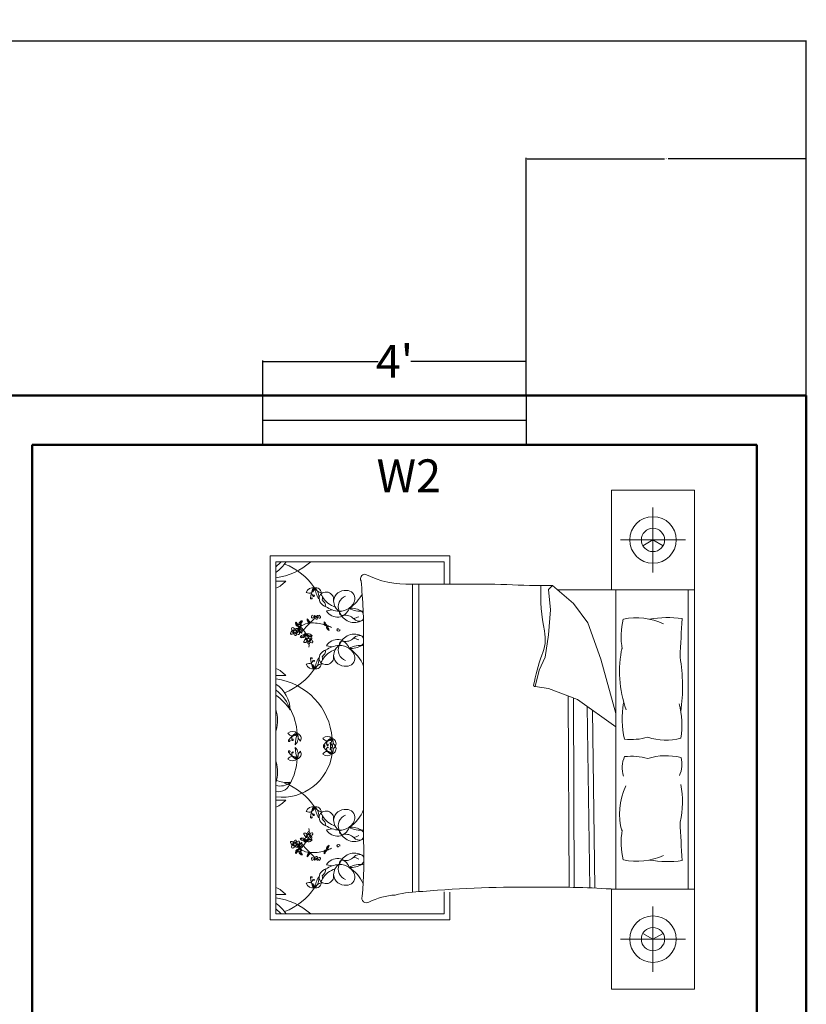
# Model space of a CAD drawing. Units: inches. Extents: x -173 to 545, y -746 to 104.
# Tile 32 of 32: x 359 to 502, y -94 to 85. Entities that reach past the tile are written whole.
import ezdxf

# ---------------------------------------------------------------- set-up
doc = ezdxf.new("R2010")
doc.units = ezdxf.units.IN
doc.header["$MEASUREMENT"] = 0
for name, color, linetype, lineweight in [('A-ANNO-DIMS', 2, 'Continuous', 18), ('A-ANNO-TEXT', 7, 'Continuous', 18), ('A-FURN', 8, 'Continuous', 18), ('A-GLAZ', 3, 'Continuous', 25), ('A-WALL', 7, 'Continuous', 50)]:
    doc.layers.add(name, color=color, linetype=linetype, lineweight=lineweight)
doc.styles.get("Standard").update_dxf_attribs({"font": 'arial.ttf'})
doc.dimstyles.get("Standard").update_dxf_attribs({"dimtxt": 0.18, "dimasz": 0.18, "dimexe": 0.18, "dimexo": 0.0625, "dimgap": 0.09, "dimtad": 0, "dimtih": 1, "dimtoh": 1, "dimdec": 0, "dimzin": 0, "dimdsep": 46, "dimlunit": 3, "dimtxsty": 'Standard', "dimcen": 0.09, "dimadec": 0, "dimazin": 0, "dimtfac": 1, "dimtdec": 0, "dimtofl": 0, "dimtmove": 0, "dimatfit": 3, "dimfxl": 1, "dimtolj": 1, "dimtzin": 0, "dimarcsym": 0})

# ---------------------------------------------------------------- blocks, each defined once
blk = doc.blocks.new('*D10')
at = {"layer": 'A-ANNO-DIMS', "color": 0, "lineweight": -2, "transparency": 16777216}
for p, q in [((402.8, 16.7), (402.8, 23.05)), ((402.98, 22.87), (423.83, 22.87)), ((450.62, 22.87), (429.77, 22.87)), ((450.8, 16.7), (450.8, 23.05))]:
    blk.add_line(p, q, dxfattribs=at)
at = {"layer": 'A-ANNO-DIMS', "color": 0, "transparency": 16777216}
for points in [[(402.98, 22.9), (402.98, 22.84), (402.8, 22.87)], [(450.62, 22.9), (450.62, 22.84), (450.8, 22.87)]]:
    blk.add_solid(points, dxfattribs=at)
at = {"layer": 'Defpoints', "color": 0, "transparency": 16777216}
for p in [(450.8, 22.87), (402.8, 16.64), (450.8, 16.64)]:
    blk.add_point(p, dxfattribs=at)
at = {"layer": 'A-ANNO-DIMS', "color": 0, "transparency": 16777216, "insert": (426.8, 22.87), "char_height": 6, "attachment_point": 5}
blk.add_mtext("\\A1;4'", dxfattribs=at)
blk = doc.blocks.new('*D23')
at = {"layer": 'A-ANNO-DIMS', "color": 0, "lineweight": -2, "transparency": 16777216}
for p, q in [((24.3, 16.7), (24.3, 81.33)), ((24.48, 81.15), (250.33, 81.15)), ((501.62, 81.15), (275.78, 81.15)), ((501.8, 16.7), (501.8, 81.33))]:
    blk.add_line(p, q, dxfattribs=at)
at = {"layer": 'A-ANNO-DIMS', "color": 0, "transparency": 16777216}
for points in [[(24.48, 81.18), (24.48, 81.12), (24.3, 81.15)], [(501.62, 81.18), (501.62, 81.12), (501.8, 81.15)]]:
    blk.add_solid(points, dxfattribs=at)
at = {"layer": 'Defpoints', "color": 0, "transparency": 16777216}
for p in [(501.8, 81.15), (24.3, 16.64), (501.8, 16.64)]:
    blk.add_point(p, dxfattribs=at)
at = {"layer": 'A-ANNO-DIMS', "color": 0, "transparency": 16777216, "insert": (263.05, 81.15), "char_height": 6, "attachment_point": 5}
blk.add_mtext('\\A1;39\'-10"', dxfattribs=at)
blk = doc.blocks.new('BED-SUITE-LARGE')
for p, q in [((77.28, 90.87), (77.28, 0)), ((69.71, 75.85), (69.71, 87.72)), ((63.77, 81.79), (75.65, 81.79)), ((0, 78.88), (32.74, 78.88)), ((0, 12.63), (0, 78.88)), ((1.05, 77.83), (1.05, 13.68)), ((31.68, 77.83), (1.05, 77.83)), ((31.68, 73.74), (31.68, 77.83)), ((32.74, 78.88), (32.74, 73.74)), ((25.93, 17.68), (25.93, 73.75)), ((27.07, 17.76), (27.07, 73.75)), ((50.66, 72.78), (51.39, 73.51)), ((51.02, 69.09), (50.66, 72.78)), ((51.39, 73.51), (55.25, 70.2)), ((77.28, 72.7), (52.34, 72.7)), ((62.92, 72.7), (62.92, 18.17)), ((76.12, 18.17), (76.12, 72.7)), ((55.25, 70.2), (57.83, 66.7)), ((10.27, 68.87), (11.29, 69.07)), ((50.66, 64.49), (51.02, 69.09)), ((57.83, 66.7), (60.22, 60.08)), ((17.01, 26.99), (17.01, 63.88)), ((50.1, 60.44), (50.66, 64.49)), ((10.27, 62.52), (11.29, 62.32)), ((49, 58.05), (50.1, 60.44)), ((60.22, 60.08), (62.92, 50.17)), ((48.26, 55.11), (49, 58.05)), ((50.66, 54.74), (48.26, 55.11)), ((55.99, 52.71), (50.66, 54.74)), ((54.42, 18.5), (54.28, 53.36)), ((55.35, 18.5), (55.22, 53.01)), ((62.92, 47.73), (55.99, 52.71)), ((58.21, 18.45), (57.75, 51.45)), ((59.15, 18.42), (58.69, 50.77)), ((10.27, 28.99), (11.29, 29.19)), ((10.27, 22.64), (11.29, 22.44)), ((31.68, 13.68), (31.68, 17.69)), ((32.74, 17.67), (32.74, 12.63)), ((69.71, 15.02), (69.71, 3.15)), ((32.74, 12.63), (0, 12.63)), ((1.05, 13.68), (31.68, 13.68)), ((63.77, 9.09), (75.65, 9.09))]:
    blk.add_line(p, q)
for points in [[(62.14, 72.7), (62.14, 90.87), (77.28, 90.87)], [(69.71, 81.79), (67.87, 80.73)], [(69.71, 81.79), (71.55, 80.73)], [(77.28, 18.17), (62.14, 18.17), (62.14, 0), (77.28, 0)], [(69.71, 9.09), (67.87, 10.15)], [(69.71, 9.09), (71.55, 10.15)]]:
    blk.add_lwpolyline(points)
for points in [[(43.07, 73.7, 0.001242), (25.83, 73.75, -0.127202), (17.23, 75.57)], [(75.02, 67.48, 0.074897), (69.08, 67.37, -0.472817)], [(68.75, 45.86, 0.14099), (74.8, 45.68, 0.235245)], [(68.75, 41.98, -0.14099), (74.8, 42.16, -0.235245)], [(75.02, 23.39, -0.074897), (69.08, 23.5, 0.472817)], [(27.78, 17.79, 0.056112), (22.78, 17.13, 0.095341), (17.97, 15.85)]]:
    blk.add_lwpolyline(points, format="xyb")
for centre, radius in [((69.71, 81.79), 4.24), ((69.71, 81.79), 2.12), ((4.53, 65.13), 0.231), ((6.97, 63.62), 0.231), ((6.97, 27.89), 0.231), ((4.53, 26.37), 0.231), ((69.71, 9.09), 4.24), ((69.71, 9.09), 2.12)]:
    blk.add_circle(centre, radius)
for centre, radius, start, end in [((-3.21, 82.79), 7.21, 306.3036, 316.4814), ((-2.13, 80.71), 5.78, 303.4617, 330.1116), ((-0.55, 86.66), 11.87, 277.745, 311.8856), ((-1.72, 66.36), 11.87, 34.3865, 68.5908), ((17.29, 74.73), 0.838, 93.98, 207.3412), ((-0.8, 77.47), 4.82, 292.5547, 318.9546), ((1.8, 90.69), 16.42, 267.4081, 273.6519), ((-77.59, 64.97), 94.6, 359.3433, 5.6887), ((49.13, 156.83), 83.35, 265.8294, 271.553), ((7.79, 71.77), 1.32, 77.7115, 159.0387), ((7.08, 73.09), 0.991, 238.4633, 358.2869), ((10.33, 71.08), 3, 138.8402, 177.9352), ((8.52, 72.2), 0.971, 117.6827, 223.7762), ((7.92, 71.62), 0.128, 223.7762, 159.7183), ((8.31, 72.1), 0.984, 2.9516, 103.728), ((16.18, 74.86), 8.3, 192.5173, 207.1824), ((6.98, 71.54), 1.88, 345.4653, 54.2343), ((9.8, 74.12), 2.03, 211.3827, 255.2969), ((10.19, 70.95), 1.36, 350.264, 160.8688), ((8.71, 71.23), 0.836, 333.9755, 53.2681), ((13.69, 70.45), 2.17, 84.9449, 172.8857), ((13.91, 71.08), 1.53, 354.4856, 91.0538), ((10.61, 75.09), 6.88, 303.6671, 333.2997), ((83.57, 71.96), 34.3, 177.4519, 191.3392), ((7.48, 71.19), 0.147, 177.9352, 11.4834), ((7.56, 71.2), 0.0716, 11.4834, 127.9409), ((10.6, 71.28), 1.7, 175.969, 254.3045), ((8.34, 69.44), 1.81, 6.1662, 51.5825), ((13.19, 73.65), 4.29, 211.2614, 251.7045), ((14.17, 70.83), 2.64, 182.3591, 234.0401), ((14.51, 69.6), 2.11, 111.5819, 201.4221), ((12.78, 71.55), 2.73, 265.2933, 346.921), ((12.85, 73.69), 4.88, 236.2883, 266.5076), ((12.22, 70), 2.26, 209.9085, 343.1337), ((13.17, 68.57), 0.564, 167.3041, 285.1471), ((14.7, 65.87), 3.5, 122.7011, 126.3445), ((15.36, 69.65), 2.9, 199.2822, 299.1751), ((16.34, 72.56), 3.76, 238.8218, 279.1554), ((14.7, 65.87), 3.5, 55.785, 94.7304), ((16, 67.9), 1.09, 30.0293, 52.325), ((4.87, 66.63), 0.258, 124.3538, 214.3923), ((5.25, 66.59), 0.602, 190.3057, 287.1958), ((5.42, 66.8), 0.7, 176.9701, 248.2913), ((10.42, 70.49), 6.76, 212.6784, 216.3746), ((5.19, 66.64), 0.268, 216.3746, 291.7548), ((5.83, 66.45), 0.602, 122.8155, 187.3992), ((5.36, 66.2), 0.202, 289.3605, 111.7548), ((6.09, 66.37), 0.7, 109.4799, 177.6828), ((5.72, 66.82), 0.258, 56.8636, 146.9021), ((5.85, 66.53), 0.268, 148.8844, 224.2646), ((11.41, 63.17), 6.76, 145.1882, 148.8844), ((7.56, 62.88), 3.77, 94.756, 119.2041), ((15.59, 57.45), 12.42, 132.2412, 142.1744), ((9.32, 67.33), 2.56, 178.3264, 187.1302), ((6.55, 66.98), 0.477, 11.3256, 64.4621), ((8.17, 67.67), 1.44, 190.2588, 210.656), ((7.21, 67.08), 0.436, 188.3432, 274.2869), ((7.59, 67.32), 0.762, 210.656, 242.6341), ((8.17, 67.98), 1.46, 218.2101, 226.3071), ((7.09, 66.75), 0.185, 325.7657, 67.4417), ((1.34, 72.94), 8.63, 313.1541, 322.0459), ((7.74, 59.14), 7.53, 73.5842, 93.8277), ((7.69, 67.76), 0.178, 142.4737, 265.053), ((7.92, 67.79), 0.382, 127.7621, 169.0403), ((7.72, 68.11), 0.538, 265.053, 338.3618), ((8.43, 67.38), 0.703, 113.4276, 137.6104), ((8.35, 68.11), 0.231, 183.2768, 356.7232), ((8.52, 67.69), 0.379, 139.7889, 227.6792), ((8.4, 67.56), 0.199, 227.6792, 350.3487), ((7.63, 67.69), 0.758, 353.0852, 15.7171), ((8.12, 67.6), 0.478, 350.3487, 43.6538), ((9.01, 68.1), 0.557, 198.7263, 262.5032), ((8.57, 67.84), 0.221, 1.1081, 91.8675), ((8.71, 67.79), 0.386, 11.5637, 52.6358), ((8.98, 67.72), 0.179, 255.2356, 54.9248), ((12.38, 66.79), 2.56, 178.3264, 187.1302), ((9.61, 66.44), 0.477, 11.3256, 64.4621), ((11.23, 67.12), 1.44, 190.2588, 210.656), ((10.27, 66.54), 0.436, 188.3432, 274.2869), ((10.65, 66.78), 0.762, 210.656, 242.6341), ((11.23, 67.43), 1.46, 218.2101, 226.3071), ((10.15, 66.21), 0.185, 325.7657, 67.4417), ((13.81, 66.22), 1.86, 41.5653, 105.1471), ((14.83, 70.08), 2.61, 277.436, 299.9149), ((16.22, 68.36), 1.36, 221.5653, 293.8354), ((16, 67.9), 1.09, 314.4517, 333.558), ((76.08, 64.24), 12.18, 165.1039, 191.0369), ((66.7, 55.9), 11.71, 65.1316, 101.7583), ((939.83, 17.39), 866.26, 176.68521, 177.14978), ((3.87, 64.78), 0.178, 142.4737, 265.053), ((4.11, 64.82), 0.382, 61.2196, 169.0403), ((3.9, 65.14), 0.538, 265.053, 338.3618), ((4.36, 65.61), 0.457, 157.4086, 261.4386), ((4.1, 65.62), 0.229, 58.0499, 135.6268), ((4.61, 64.41), 0.703, 113.4276, 137.6104), ((4.34, 65.48), 0.153, 172.906, 277.132), ((3.83, 65.2), 0.73, 14.7558, 58.0499), ((4.7, 64.72), 0.379, 139.7889, 227.6792), ((4.86, 65.39), 0.316, 36.1046, 181.4281), ((3.81, 64.72), 0.758, 353.0852, 15.7171), ((4.31, 64.63), 0.478, 350.3487, 43.6538), ((4.67, 65.64), 0.319, 270.0645, 331.1507), ((4.94, 65.56), 0.364, 221.8413, 265.7877), ((5.19, 65.12), 0.557, 198.7263, 262.5032), ((4.75, 64.86), 0.221, 1.1081, 91.8675), ((4.94, 65.42), 0.227, 263.7526, 41.7054), ((4.89, 64.81), 0.386, 11.5637, 86.365), ((7.56, 62.88), 3.77, 124.0033, 132.4917), ((5.17, 64.75), 0.179, 255.2356, 54.9248), ((3.67, 62.41), 4.03, 63.7819, 68.2913), ((5.83, 65.51), 0.641, 128.3208, 208.8162), ((5.94, 65.56), 0.766, 207.7043, 254.3516), ((5.51, 66.2), 0.202, 221.8703, 44.2646), ((6.43, 65.62), 1.05, 157.2305, 229.0635), ((6.07, 65.96), 0.621, 174.4544, 220.6188), ((5.44, 65.12), 1.05, 270.278, 342.111), ((2.54, 62.5), 4.53, 30.544, 49.818), ((5.04, 65.07), 0.746, 340.0041, 40.6188), ((5.94, 65.15), 0.621, 278.7227, 324.8872), ((5.83, 64.65), 0.641, 290.5253, 358.5375), ((7.08, 64.83), 0.641, 182.8499, 266.1226), ((6.83, 65.28), 0.621, 231.7607, 277.9252), ((7.32, 65.39), 1.05, 214.5369, 286.3699), ((7.02, 63.93), 0.746, 37.3105, 97.9252), ((10.67, 65.87), 0.436, 147.5332, 233.4768), ((11.06, 66.09), 0.762, 179.1859, 211.164), ((10.32, 65.92), 0.185, 354.3784, 96.0543), ((7.74, 59.14), 7.53, 63.0032, 69.8941), ((11.64, 66.44), 1.44, 211.164, 231.5612), ((11.89, 67.61), 2.56, 234.6898, 243.4936), ((11.91, 66.29), 1.46, 195.5129, 203.6099), ((10.27, 65.34), 0.477, 357.3579, 50.4944), ((12.32, 65.43), 0.175, 12.7051, 190.4384), ((12.43, 65.45), 0.285, 190.4384, 10.4136), ((15.36, 61.74), 2.9, 60.8249, 160.7178), ((42.69, 63.76), 7.4, 336.2616, 11.3392), ((4.58, 64.58), 0.199, 227.6792, 350.3487), ((6.15, 63.8), 0.746, 98.7227, 159.3375), ((5.77, 64.76), 0.766, 244.9899, 291.6373), ((6.31, 63.27), 0.178, 142.4737, 265.053), ((6.54, 63.31), 0.382, 61.2196, 169.0403), ((6.34, 63.63), 0.538, 265.053, 338.3618), ((6.8, 64.09), 0.457, 157.4086, 261.4386), ((6.54, 64.11), 0.229, 58.0499, 135.6268), ((7.05, 62.89), 0.703, 113.4276, 137.6104), ((6.78, 63.96), 0.153, 172.906, 277.132), ((6.27, 63.68), 0.73, 14.7558, 58.0499), ((2.54, 62.5), 4.53, 23.0501, 23.8477), ((7.14, 63.2), 0.379, 139.7889, 227.6792), ((7.02, 63.07), 0.199, 227.6792, 350.3487), ((7.3, 63.88), 0.316, 36.1046, 181.4281), ((6.25, 63.21), 0.758, 353.0852, 15.7171), ((7.11, 64.95), 0.766, 265.0106, 311.658), ((2.54, 62.5), 4.53, 357.1071, 4.7585), ((6.75, 63.12), 0.478, 350.3487, 43.6538), ((7.11, 64.12), 0.319, 270.0645, 331.1507), ((7.38, 64.05), 0.364, 221.8413, 265.7877), ((7.63, 63.61), 0.557, 198.7263, 262.5032), ((7.19, 63.35), 0.221, 1.1081, 91.8675), ((7.38, 63.91), 0.227, 263.7526, 41.7054), ((7.33, 63.3), 0.386, 11.5637, 86.365), ((7.61, 63.23), 0.179, 255.2356, 54.9248), ((12.22, 61.39), 2.26, 16.8663, 150.0915), ((13.17, 62.82), 0.564, 74.8529, 192.6959), ((13.81, 65.17), 1.86, 254.8529, 318.4347), ((14.83, 61.31), 2.61, 60.0851, 82.564), ((16.22, 63.03), 1.36, 66.1646, 138.4347), ((16, 63.49), 1.09, 307.675, 336.7144), ((16, 63.49), 1.09, 23.229, 45.5483), ((10.6, 60.11), 1.7, 105.6955, 184.031), ((8.34, 61.95), 1.81, 308.4175, 353.8338), ((13.19, 57.74), 4.29, 108.2955, 148.7386), ((12.85, 57.7), 4.88, 93.4924, 123.7117), ((14.17, 60.56), 2.64, 125.9599, 177.6409), ((14.51, 61.79), 2.11, 158.5779, 248.4181), ((12.78, 59.84), 2.73, 13.079, 94.7067), ((14.7, 65.52), 3.5, 233.6555, 237.2989), ((16.34, 58.83), 3.76, 79.7133, 121.1782), ((14.7, 65.52), 3.5, 265.2696, 304.215), ((10.61, 56.3), 6.88, 21.4941, 56.3329), ((84.74, 57.83), 21.12, 168.0397, 199.2615), ((7.08, 58.3), 0.991, 1.7131, 121.5367), ((7.48, 60.2), 0.147, 348.5166, 182.0648), ((10.33, 60.31), 3, 182.0648, 221.1598), ((7.56, 60.19), 0.0716, 232.0591, 348.5166), ((8.52, 59.19), 0.971, 136.2238, 242.3173), ((7.97, 59.76), 0.0774, 200.2667, 136.2271), ((6.98, 59.85), 1.88, 305.7657, 14.5347), ((16.18, 56.53), 8.3, 152.8176, 167.4827), ((8.31, 59.29), 0.984, 256.272, 357.0484), ((9.8, 57.27), 2.03, 104.7031, 148.6173), ((10.19, 60.44), 1.36, 199.1312, 9.736), ((8.71, 60.16), 0.836, 306.7319, 26.0245), ((13.69, 60.94), 2.17, 187.1143, 275.0551), ((13.91, 60.31), 1.53, 268.9462, 5.5144), ((82.6, 48.8), 35.24, 160.1194, 169.3383), ((42.13, 55.03), 32.96, 352.2196, 9.497), ((-0.8, 53.92), 4.82, 41.0454, 67.4453), ((-1.72, 65.03), 11.87, 291.4092, 325.6135), ((7.79, 59.62), 1.32, 200.9613, 282.2885), ((1.8, 40.7), 16.42, 86.3481, 92.5919), ((-0.55, 44.73), 11.87, 4.4623, 82.255), ((-2.13, 50.68), 5.78, 1.272, 56.5383), ((-3.21, 48.6), 7.21, 17.8504, 53.6964), ((48.19, 55.31), 0.219, 178.8623, 289.7536), ((-5.24, 44.82), 10.72, 34.0123, 54.053), ((80.12, 49.28), 16.03, 169.8617, 193.6238), ((-5.19, 48.96), 6.53, 343.5431, 17.0202), ((-6.9, 45.64), 11.87, 4.4623, 27.4146), ((58.79, 48.07), 16.19, 351.5249, 13.96), ((-8.55, 46.37), 9.65, 4.3787, 5.6357), ((-15.16, 41.29), 17.24, 19.7217, 19.9028), ((4.04, 45.59), 1.32, 47.7873, 129.1145), ((4.09, 47.08), 0.991, 208.5391, 328.3627), ((3.48, 45.23), 0.147, 148.011, 341.5592), ((5.9, 43.72), 3, 108.9159, 148.011), ((3.55, 45.21), 0.0716, 341.5592, 98.0167), ((4.89, 45.59), 0.971, 87.7585, 193.852), ((4.07, 45.39), 0.128, 193.852, 129.9245), ((12.85, 44.08), 8.3, 162.593, 177.2582), ((3.22, 45.79), 1.88, 315.5411, 24.3101), ((6.96, 46.61), 2.03, 181.4585, 225.3727), ((4.65, 45.62), 0.984, 333.0274, 73.8037), ((10.4, 44.68), 1.32, 47.7873, 129.1145), ((10.44, 46.17), 0.991, 208.5391, 328.3627), ((12.26, 42.81), 3, 108.9159, 148.011), ((11.25, 44.68), 0.971, 87.7585, 193.852), ((9.58, 44.88), 1.88, 315.5411, 24.3101), ((19.21, 43.17), 8.3, 162.593, 177.2582), ((9.58, 43.6), 1.88, 335.6899, 44.4589), ((19.21, 45.31), 8.3, 182.7418, 197.407), ((11.01, 44.71), 0.984, 333.0274, 73.8037), ((13.31, 45.7), 2.03, 181.4585, 225.3727), ((65.71, 56.57), 11.13, 264.0129, 285.8293), ((3.48, 43.24), 0.147, 18.4408, 211.989), ((5.9, 44.75), 3, 211.989, 251.0841), ((3.55, 43.27), 0.0716, 261.9833, 18.4408), ((4.89, 42.89), 0.971, 166.148, 272.2415), ((4.12, 43.1), 0.0774, 230.1909, 166.0209), ((12.85, 44.4), 8.3, 182.7418, 197.407), ((3.22, 42.69), 1.88, 335.6899, 44.4589), ((6.96, 41.86), 2.03, 134.6273, 178.5415), ((4.65, 42.86), 0.984, 286.1963, 26.9726), ((10.44, 42.3), 0.991, 31.6373, 151.4609), ((9.84, 44.33), 0.147, 148.011, 341.5592), ((9.84, 44.15), 0.147, 18.4408, 211.989), ((12.26, 45.66), 3, 211.989, 251.0841), ((9.91, 44.3), 0.0716, 341.5592, 98.0167), ((9.91, 44.18), 0.0716, 261.9833, 18.4408), ((11.25, 43.79), 0.971, 166.148, 272.2415), ((10.43, 44.48), 0.128, 193.852, 129.9245), ((10.48, 44.01), 0.0774, 230.1909, 166.0209), ((11.01, 43.77), 0.984, 286.1963, 26.9726), ((13.31, 42.77), 2.03, 134.6273, 178.5415), ((2.19, 44.13), 9.18, 262.8636, 351.8197), ((-5.19, 39.52), 6.53, 342.9798, 16.4569), ((-8.55, 42.11), 9.65, 354.3643, 355.6213), ((-15.16, 47.19), 17.24, 340.0972, 340.2783), ((4.09, 41.4), 0.991, 31.6373, 151.4609), ((4.04, 42.89), 1.32, 230.8855, 312.2127), ((-6.9, 42.84), 11.87, 332.5854, 355.5377), ((10.4, 43.8), 1.32, 230.8855, 312.2127), ((68.92, 40.31), 4.82, 155.0183, 198.5407), ((65.71, 31.27), 11.13, 74.1707, 95.9871), ((70.49, 40.92), 4.5, 333.3437, 16.1026), ((3.03, 42.94), 5.31, 248.117, 276.6195), ((1.55, 38.07), 2.13, 256.3898, 349.0739), ((1.85, 39.67), 2.69, 252.8609, 311.9049), ((-1.72, 26.47), 11.87, 34.3865, 68.5908), ((75.18, 31.89), 11.57, 153.8761, 196.1746), ((59.12, 34.18), 15.97, 346.3427, 11.1841), ((1.8, 50.8), 16.42, 267.4081, 273.6519), ((-0.8, 37.59), 4.82, 292.5547, 318.9546), ((7.79, 31.89), 1.32, 77.7115, 159.0387), ((7.08, 33.21), 0.991, 238.4633, 358.2869), ((10.33, 31.2), 3, 138.8402, 177.9352), ((8.52, 32.32), 0.971, 117.6827, 223.7762), ((8.31, 32.22), 0.984, 2.9516, 103.728), ((9.8, 34.23), 2.03, 211.3827, 255.2969), ((6.98, 31.65), 1.88, 345.4653, 54.2343), ((16.18, 34.98), 8.3, 192.5173, 207.1824), ((10.19, 31.07), 1.36, 350.264, 160.8688), ((13.69, 30.57), 2.17, 84.9449, 172.8857), ((13.91, 31.2), 1.53, 354.4856, 91.0538), ((10.61, 35.2), 6.88, 303.6671, 338.5059), ((7.48, 31.3), 0.147, 177.9352, 11.4834), ((7.56, 31.32), 0.0716, 11.4834, 127.9409), ((7.92, 31.73), 0.128, 223.7762, 159.7183), ((10.6, 31.39), 1.7, 175.969, 254.3045), ((8.71, 31.35), 0.836, 333.9755, 53.2681), ((8.34, 29.56), 1.81, 6.1662, 51.5825), ((13.19, 33.77), 4.29, 211.2614, 251.7045), ((14.17, 30.94), 2.64, 182.3591, 234.0401), ((14.51, 29.71), 2.11, 111.5819, 201.4221), ((12.78, 31.67), 2.73, 265.2933, 346.921), ((2.54, 29.01), 4.53, 355.2415, 2.8929), ((12.85, 33.81), 4.88, 236.2883, 266.5076), ((12.22, 30.11), 2.26, 209.9085, 343.1337), ((13.17, 28.68), 0.564, 167.3041, 285.1471), ((14.7, 25.98), 3.5, 122.7011, 126.3445), ((15.36, 29.76), 2.9, 199.2822, 299.1751), ((16.34, 32.68), 3.76, 238.8218, 280.2867), ((14.7, 25.98), 3.5, 55.785, 94.7304), ((16, 28.02), 1.09, 23.2856, 52.325), ((76.08, 26.64), 12.18, 168.9631, 194.8961), ((939.83, 73.48), 866.26, 182.85022, 183.31479), ((3.87, 26.72), 0.178, 94.947, 217.5263), ((3.9, 26.36), 0.538, 21.6382, 94.947), ((4.7, 26.79), 0.379, 132.3208, 220.2111), ((4.58, 26.92), 0.199, 9.6513, 132.3208), ((4.31, 26.88), 0.478, 316.3462, 9.6513), ((5.19, 26.38), 0.557, 97.4968, 161.2737), ((5.17, 26.76), 0.179, 305.0752, 104.7644), ((5.77, 26.75), 0.766, 68.3627, 115.0101), ((5.44, 26.39), 1.05, 17.889, 89.722), ((6.15, 27.71), 0.746, 200.6625, 261.2773), ((5.94, 26.36), 0.621, 35.1128, 81.2773), ((5.83, 26.86), 0.641, 1.4625, 69.4747), ((6.31, 28.24), 0.178, 94.947, 217.5263), ((6.54, 28.2), 0.382, 190.9597, 298.7804), ((6.34, 27.88), 0.538, 21.6382, 94.947), ((6.8, 27.42), 0.457, 98.5614, 202.5914), ((6.54, 27.4), 0.229, 224.3732, 301.9501), ((7.08, 26.68), 0.641, 93.8774, 177.1501), ((7.32, 26.11), 1.05, 73.6301, 145.4631), ((7.05, 28.61), 0.703, 222.3896, 246.5724), ((6.78, 27.54), 0.153, 82.868, 187.094), ((6.27, 27.82), 0.73, 301.9501, 345.2442), ((2.54, 29.01), 4.53, 336.1523, 336.9499), ((7.14, 28.3), 0.379, 132.3208, 220.2111), ((7.02, 28.44), 0.199, 9.6513, 132.3208), ((7.02, 27.58), 0.746, 262.0748, 322.6895), ((6.25, 28.3), 0.758, 344.2829, 6.9148), ((7.3, 27.63), 0.316, 178.5719, 323.8954), ((7.11, 26.55), 0.766, 48.342, 94.9894), ((6.75, 28.39), 0.478, 316.3462, 9.6513), ((7.63, 27.9), 0.557, 97.4968, 161.2737), ((7.38, 27.46), 0.364, 94.2123, 138.1587), ((7.11, 27.38), 0.319, 28.8493, 89.9355), ((7.19, 28.16), 0.221, 268.1325, 358.8919), ((7.33, 28.21), 0.386, 273.635, 348.4363), ((7.38, 27.6), 0.227, 318.2946, 96.2474), ((7.61, 28.28), 0.179, 305.0752, 104.7644), ((13.81, 26.34), 1.86, 41.5653, 105.1471), ((14.83, 30.2), 2.61, 277.436, 299.9149), ((16.22, 28.48), 1.36, 221.5653, 293.8354), ((-71.37, 24.21), 88.43, 355.2402, 1.8035), ((16, 28.02), 1.09, 314.4517, 336.7144), ((4.11, 26.69), 0.382, 190.9597, 298.7804), ((4.36, 25.9), 0.457, 98.5614, 202.5914), ((4.1, 25.89), 0.229, 224.3732, 301.9501), ((4.61, 27.1), 0.703, 222.3896, 246.5724), ((4.34, 26.03), 0.153, 82.868, 187.094), ((3.83, 26.31), 0.73, 301.9501, 345.2442), ((3.81, 26.79), 0.758, 344.2829, 6.9148), ((4.86, 26.12), 0.316, 178.5719, 323.8954), ((5.25, 24.92), 0.602, 72.8042, 169.6943), ((4.94, 25.94), 0.364, 94.2123, 138.1587), ((4.67, 25.87), 0.319, 28.8493, 89.9355), ((5.42, 24.7), 0.7, 111.7087, 183.0299), ((4.75, 26.64), 0.221, 268.1325, 358.8919), ((4.89, 26.69), 0.386, 273.635, 348.4363), ((4.94, 26.08), 0.227, 318.2946, 96.2474), ((5.19, 24.87), 0.268, 68.2452, 143.6254), ((7.56, 28.62), 3.77, 227.5083, 235.9967), ((3.67, 29.1), 4.03, 291.7087, 296.2181), ((5.83, 26), 0.641, 151.1838, 231.6792), ((5.83, 25.05), 0.602, 172.6008, 237.1845), ((5.94, 25.95), 0.766, 105.6484, 152.2957), ((5.36, 25.3), 0.202, 248.2452, 70.6395), ((5.51, 25.3), 0.202, 315.7354, 138.1297), ((6.43, 25.89), 1.05, 130.9365, 202.7695), ((6.07, 25.54), 0.621, 139.3812, 185.5456), ((2.54, 29.01), 4.53, 310.182, 329.456), ((5.85, 24.98), 0.268, 135.7354, 211.1156), ((5.04, 26.43), 0.746, 319.3812, 19.9959), ((7.56, 28.62), 3.77, 240.7959, 265.244), ((15.59, 34.05), 12.42, 217.8256, 227.7588), ((6.83, 26.23), 0.621, 82.0748, 128.2393), ((7.74, 32.37), 7.53, 266.1723, 286.4158), ((11.23, 24.38), 1.44, 149.344, 169.7412), ((10.27, 24.97), 0.436, 85.7131, 171.6568), ((10.65, 24.73), 0.762, 117.3659, 149.344), ((11.23, 24.07), 1.46, 133.6929, 141.7899), ((10.15, 25.3), 0.185, 292.5583, 34.2343), ((10.67, 25.64), 0.436, 126.5232, 212.4668), ((11.06, 25.41), 0.762, 148.836, 180.8141), ((10.32, 25.59), 0.185, 263.9457, 5.6216), ((7.74, 32.37), 7.53, 290.1059, 296.9968), ((11.64, 25.06), 1.44, 128.4388, 148.836), ((11.89, 23.9), 2.56, 116.5064, 125.3102), ((11.91, 25.21), 1.46, 156.3901, 164.4871), ((10.27, 26.17), 0.477, 309.5056, 2.6421), ((12.32, 26.07), 0.175, 169.5616, 347.2949), ((12.43, 26.05), 0.285, 349.5864, 169.5616), ((4.87, 24.88), 0.258, 145.6077, 235.6462), ((10.42, 21.02), 6.76, 143.6254, 147.3216), ((6.09, 25.13), 0.7, 182.3172, 250.5201), ((5.72, 24.69), 0.258, 213.0979, 303.1364), ((11.41, 28.33), 6.76, 211.1156, 214.8118), ((8.17, 23.84), 1.44, 149.344, 169.7412), ((9.32, 24.17), 2.56, 172.8698, 181.6736), ((6.55, 24.53), 0.477, 295.5379, 348.6744), ((7.21, 24.43), 0.436, 85.7131, 171.6568), ((7.59, 24.19), 0.762, 117.3659, 149.344), ((8.17, 23.53), 1.46, 133.6929, 141.7899), ((7.09, 24.76), 0.185, 292.5583, 34.2343), ((1.34, 18.57), 8.63, 37.9541, 46.8459), ((7.69, 23.75), 0.178, 94.947, 217.5263), ((7.92, 23.72), 0.382, 190.9597, 232.2379), ((7.72, 23.39), 0.538, 21.6382, 94.947), ((8.43, 24.13), 0.703, 222.3896, 246.5724), ((8.35, 23.4), 0.231, 3.2768, 176.7232), ((8.52, 23.82), 0.379, 132.3208, 220.2111), ((8.4, 23.95), 0.199, 9.6513, 132.3208), ((7.63, 23.81), 0.758, 344.2829, 6.9148), ((8.12, 23.9), 0.478, 316.3462, 9.6513), ((9.01, 23.41), 0.557, 97.4968, 161.2737), ((8.57, 23.67), 0.221, 268.1325, 358.8919), ((8.98, 23.79), 0.179, 305.0752, 104.7644), ((8.71, 23.72), 0.386, 307.3642, 348.4363), ((12.38, 24.71), 2.56, 172.8698, 181.6736), ((9.61, 25.07), 0.477, 295.5379, 348.6744), ((12.22, 21.51), 2.26, 16.8663, 150.0915), ((13.17, 22.94), 0.564, 74.8529, 192.6959), ((15.36, 21.86), 2.9, 60.8249, 160.7178), ((13.81, 25.28), 1.86, 254.8529, 318.4347), ((14.83, 21.42), 2.61, 60.0851, 82.564), ((16.22, 23.14), 1.36, 66.1646, 138.4347), ((16, 23.61), 1.09, 16.6343, 45.5483), ((66.7, 34.97), 11.71, 258.2417, 294.8684), ((10.6, 20.23), 1.7, 105.6955, 184.031), ((8.34, 22.06), 1.81, 308.4175, 353.8338), ((13.19, 17.85), 4.29, 108.2955, 148.7386), ((12.85, 17.81), 4.88, 93.4924, 123.7117), ((14.17, 20.68), 2.64, 125.9599, 177.6409), ((14.51, 21.91), 2.11, 158.5779, 248.4181), ((12.78, 19.96), 2.73, 13.079, 94.7067), ((14.7, 25.64), 3.5, 233.6555, 237.2989), ((16.34, 18.94), 3.76, 79.249, 121.1782), ((14.7, 25.64), 3.5, 265.2696, 304.215), ((10.61, 16.42), 6.88, 23.6453, 56.3329), ((16, 23.61), 1.09, 307.675, 342.5814), ((7.48, 20.32), 0.147, 348.5166, 182.0648), ((10.33, 20.42), 3, 182.0648, 221.1598), ((7.56, 20.3), 0.0716, 232.0591, 348.5166), ((8.52, 19.31), 0.971, 136.2238, 242.3173), ((7.97, 19.88), 0.0774, 200.2667, 136.2271), ((16.18, 16.65), 8.3, 152.8176, 167.4827), ((6.98, 19.97), 1.88, 305.7657, 14.5347), ((10.19, 20.56), 1.36, 199.1312, 9.736), ((8.71, 20.28), 0.836, 306.7319, 26.0245), ((13.69, 21.06), 2.17, 187.1143, 275.0551), ((13.91, 20.43), 1.53, 268.9462, 5.5144), ((-0.8, 14.04), 4.82, 41.0454, 67.4453), ((-1.72, 25.15), 11.87, 291.4092, 325.6135), ((7.08, 18.42), 0.991, 1.7131, 121.5367), ((7.79, 19.73), 1.32, 200.9613, 282.2885), ((9.8, 17.39), 2.03, 104.7031, 148.6173), ((8.31, 19.4), 0.984, 256.272, 357.0484), ((45.88, -194.44), 213, 89.1145, 94.8735), ((51.82, -144.73), 163.28, 86.1, 90.9282), ((1.8, 0.82), 16.42, 86.3481, 92.5919), ((-0.55, 4.85), 11.87, 48.1144, 82.255), ((17.51, 16.54), 0.828, 156.5219, 303.8264), ((-2.13, 10.8), 5.78, 29.8884, 56.5383), ((-3.21, 8.72), 7.21, 43.5186, 53.6964)]:
    blk.add_arc(centre, radius, start, end)
blk = doc.blocks.new('WINDOW-48')
for p, q in [((0, 9), (48, 9)), ((0, 0), (0, 9)), ((48, 9), (48, 0)), ((0, 4.5), (48, 4.5)), ((48, 0), (0, 0))]:
    blk.add_line(p, q)
blk = doc.blocks.new('*D79')
at = {"layer": 'A-ANNO-DIMS', "color": 0, "lineweight": -2, "transparency": 16777216}
for p, q in [((450.8, 16.7), (450.8, 59.92)), ((450.98, 59.74), (475.97, 59.74)), ((501.62, 59.74), (476.63, 59.74)), ((501.8, 16.7), (501.8, 59.92))]:
    blk.add_line(p, q, dxfattribs=at)
at = {"layer": 'A-ANNO-DIMS', "color": 0, "transparency": 16777216}
for points in [[(450.98, 59.77), (450.98, 59.71), (450.8, 59.74)], [(501.62, 59.77), (501.62, 59.71), (501.8, 59.74)]]:
    blk.add_solid(points, dxfattribs=at)
at = {"layer": 'Defpoints', "color": 0, "transparency": 16777216}
for p in [(501.8, 59.74), (450.8, 16.64), (501.8, 16.64)]:
    blk.add_point(p, dxfattribs=at)
at = {"layer": 'A-ANNO-DIMS', "color": 0, "transparency": 16777216, "insert": (476.3, 59.74), "char_height": 0.18, "attachment_point": 5}
blk.add_mtext('\\A1;4\'-3"', dxfattribs=at)

msp = doc.modelspace()

# ---------------------------------------------------------------- linework, layer by layer
at = {"layer": 'A-WALL'}
for p, q in [((24.3, 16.64), (501.8, 16.64)), ((501.8, 7.64), (501.8, 16.64)), ((360.8, 7.64), (360.8, -128.86)), ((360.8, 7.64), (492.8, 7.64)), ((492.8, 7.64), (492.8, -124.36)), ((501.8, 7.64), (501.8, -697.36))]:
    msp.add_line(p, q, dxfattribs=at)

# ---------------------------------------------------------------- block references
at = {"layer": 'A-FURN'}
msp.add_blockref('BED-SUITE-LARGE', (404.17, -91.45), dxfattribs=at)
at = {"layer": 'A-GLAZ'}
msp.add_blockref('WINDOW-48', (402.8, 7.64), dxfattribs=at)

# ---------------------------------------------------------------- texts
at = {"layer": 'A-ANNO-TEXT', "insert": (423.55, 5.02), "char_height": 6, "attachment_point": 1}
msp.add_mtext('W2', dxfattribs=at)

# ---------------------------------------------------------------- dimensions: what is measured, and where the dimension line sits
at = {"layer": 'A-ANNO-DIMS'}
for base, p1, p2, override, picture, middle in [((501.80136521, 81.15311648), (24.30136521, 16.63801408), (501.80136521, 16.63801408), {"dimtxt": 6, "dimclrd": 0, "dimclre": 0, "dimclrt": 0}, '*D23', (263.05136521, 81.15311648)), ((501.8, 59.74), (450.8, 16.64), (501.8, 16.64), {"dimdec": 1, "dimlfac": 1, "dimrnd": 0, "dimzin": 1, "dimdsep": 46, "dimlunit": 4, "dimfrac": 2}, '*D79', (476.3, 59.74)), ((450.8, 22.87), (402.8, 16.64), (450.8, 16.64), {"dimtxt": 6, "dimclrd": 0, "dimclre": 0, "dimclrt": 0}, '*D10', (426.8, 22.87))]:
    dim = msp.add_linear_dim(base=base, p1=p1, p2=p2, dimstyle='Standard', override=override, dxfattribs=at)
    dim.commit()
    dim.dimension.update_dxf_attribs({"geometry": picture, "text_midpoint": middle})

doc.saveas('drawing.dxf')
